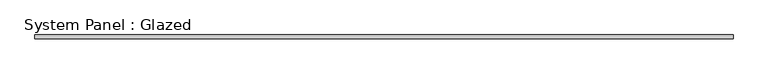
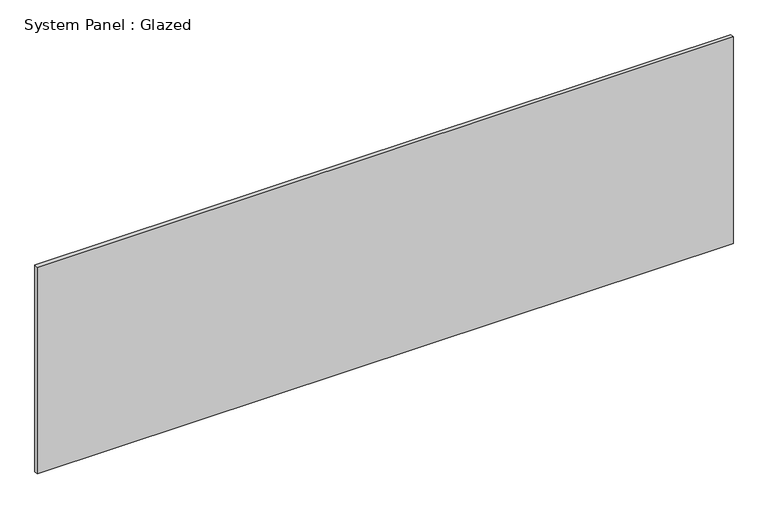
"""IFC4 building model written with IfcOpenShell, lengths in millimetres: plate geometry, System Panel : Glazed."""

from ifc_helpers import new_model, si_unit, origin, origin_with_axes, place, context, project, spatial, polyline, outline, extrude, source, transform, mapped, element, save


def system_panel_glazed_4760f0d8(model_context):
    return source(origin(), model_context, "Body", "SweptSolid", [
        extrude(outline(polyline([(2425.7, 19.05), (-2425.7, 19.05), (-2425.7, 44.45), (2425.7, 44.45), (2425.7, 19.05)])), origin_with_axes(), (0.0, 0.0, 1.0), 1524.0),
    ])


if __name__ == "__main__":
    model = new_model("IFC4")
    model_context = context("Model", 3, world=origin())
    ifc_project = project(units=[si_unit("LENGTHUNIT", "METRE", prefix="MILLI")], contexts=[model_context])
    site = spatial("IfcSite", under=ifc_project)
    building = spatial("IfcBuilding", under=site)
    placement = place(None, origin())
    system_panel_glazed_shape = system_panel_glazed_4760f0d8(model_context)
    element("IfcPlate", 1, ObjectType="System Panel : Glazed", at=placement, inside=building, context=model_context, shape_type="MappedRepresentation", body=[
        mapped(system_panel_glazed_shape, transform((0.0, 0.0, 0.0), x_axis=(1.0, 0.0, 0.0), y_axis=(0.0, 1.0, 0.0), z_axis=(0.0, 0.0, 1.0))),
    ])
    save(model, "model.ifc")

# Revit data of these elements
# Type "System Panel : Glazed"
#   Construction Type Id = "GSP4R"
#   Analytic Construction = "1/8 in Pilkington single glazing"
#   Visual Light Transmittance = 0.9
#   Solar Heat Gain Coefficient = 0.86
#   Heat Transfer Coefficient (U) = 1.18115 BTU/(h·ft²·°F)
# Element 1 (IfcPlate, "System Panel : Glazed")
#   Materials on its faces: "Glass"
# Materials
#   "Glass": class "Glass", colour RGB 0 128 192, transparency 0.75, Description = "Soda Lime Glass", Cost = 0
